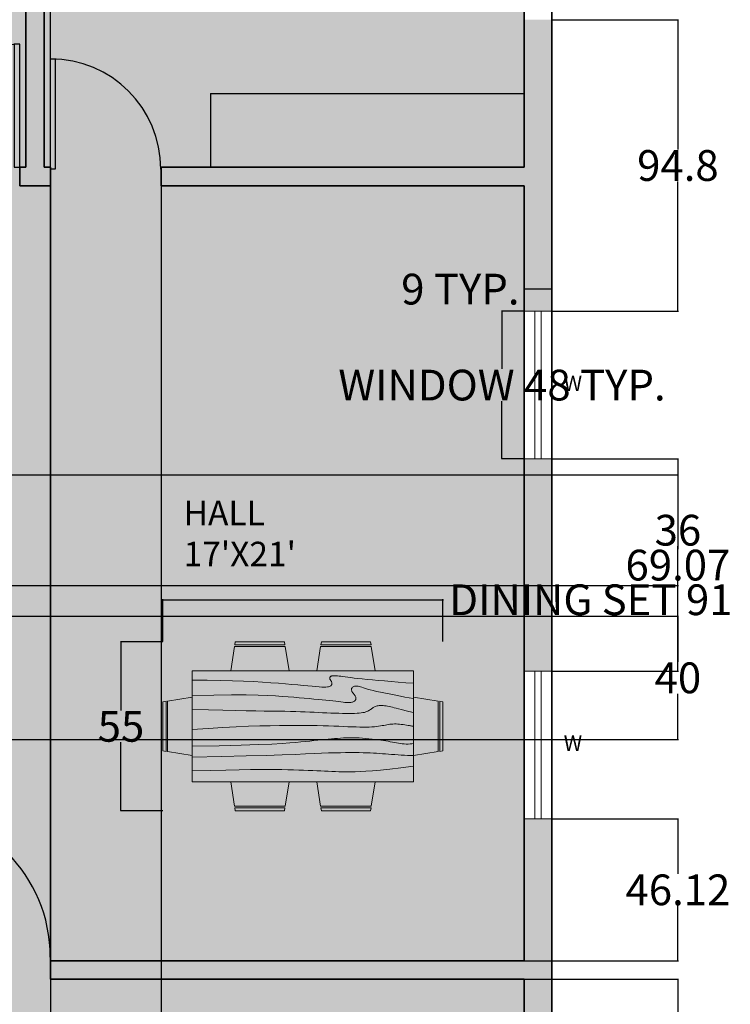
# Model space of a CAD drawing. Units: inches. Extents: x 286 to 756, y 360 to 1175.
# Tile 3 of 4: x 525 to 756, y 649 to 969. Entities that reach past the tile are written whole.
import ezdxf

# ---------------------------------------------------------------- set-up
doc = ezdxf.new("R2010")
doc.units = ezdxf.units.IN
doc.header["$MEASUREMENT"] = 0
for name, color, linetype, lineweight in [('A-ANNO-DIMS', 2, 'Continuous', 18), ('A-ANNO-TEXT', 7, 'Continuous', 18), ('A-AREA-IDEN', 7, 'Continuous', 18), ('A-FLOR-CASE', 8, 'Continuous', 25), ('A-GLAZ', 4, 'Continuous', 18), ('A-WALL', 7, 'Continuous', 35), ('DOOR', 6, 'Continuous', 25), ('FUR', 8, 'Continuous', 18)]:
    doc.layers.add(name, color=color, linetype=linetype, lineweight=lineweight)
for name, color, linetype, lineweight, true_color in [('A-FLOR-CASE-PATT', 30, 'Continuous', 13, 0xf8991e), ('A-FLOR-PATT', 9, 'Continuous', 13, 0xc7c8ca), ('A-WALL-PATT', 18, 'Continuous', 13, 0x000000)]:
    doc.layers.add(name, color=color, linetype=linetype, lineweight=lineweight, true_color=true_color)
doc.styles.get("Standard").update_dxf_attribs({"font": 'arial.ttf'})
doc.dimstyles.get("Standard").update_dxf_attribs({"dimtxt": 10, "dimasz": 0.18, "dimexe": 0.18, "dimexo": 0.0625, "dimgap": 0.09, "dimtad": 0, "dimtih": 1, "dimtoh": 1, "dimdec": 0, "dimzin": 0, "dimdsep": 46, "dimlunit": 3, "dimtxsty": 'Standard', "dimcen": 0.09, "dimadec": 0, "dimazin": 0, "dimtfac": 1, "dimtdec": 0, "dimtofl": 0, "dimtmove": 0, "dimatfit": 3, "dimfxl": 1, "dimtolj": 1, "dimtzin": 0, "dimarcsym": 0})

# ---------------------------------------------------------------- blocks, each defined once
blk = doc.blocks.new('Dining Set - 36 x 72 in.')
for p, q in [((-22.2343, 26.00059), (-23.4847, 17.99762)), ((-22.2304, 26), (-5.7608, 26)), ((-22, 27.5), (-22.1562, 26.50042)), ((-5.8416, 26.5), (-22.1534, 26.5)), ((-22, 27.5), (-6, 27.5)), ((-5.8437, 26.49966), (-6, 27.5)), ((-4.5152, 17.99762), (-5.7655, 25.99926)), ((5.7657, 26.00059), (4.5153, 17.99762)), ((5.7696, 26), (22.2392, 26)), ((6, 27.5), (5.8438, 26.50042)), ((22.1584, 26.5), (5.8466, 26.5)), ((6, 27.5), (22, 27.5)), ((22.1563, 26.49966), (22, 27.5)), ((23.4848, 17.99762), (22.2345, 25.99926)), ((36, 18), (-36, 18)), ((-36, 18), (-36, -18)), ((36, -18), (36, 18)), ((-45.5, 8), (-44.5004, 8.15617)), ((-45.5, 8), (-45.5, -8)), ((-44.5, -8.15843), (-44.5, 8.15338)), ((-44.0006, 8.23428), (-35.9976, 9.48474)), ((-44, 8.23041), (-44, -8.23915)), ((44.0006, 8.23428), (35.9976, 9.48474)), ((44, 8.23041), (44, -8.23915)), ((44.5, -8.15843), (44.5, 8.15338)), ((45.5, 8), (44.5005, 8.15617)), ((45.5, 8), (45.5, -8)), ((-44.4997, -8.15631), (-45.5, -8)), ((-35.9976, -9.48476), (-43.9993, -8.2345)), ((35.9976, -9.48476), (43.9993, -8.2345)), ((44.4997, -8.15631), (45.5, -8)), ((-36, -18), (36, -18)), ((-22.2343, -26.0006), (-23.4847, -17.99762)), ((-4.5152, -17.99762), (-5.7655, -25.99928)), ((5.7657, -26.0006), (4.5153, -17.99762)), ((23.4848, -17.99762), (22.2345, -25.99928)), ((-22.2304, -26), (-5.7608, -26)), ((-22, -27.5), (-22.1562, -26.50044)), ((-5.8416, -26.5), (-22.1534, -26.5)), ((-22, -27.5), (-6, -27.5)), ((-5.8437, -26.49967), (-6, -27.5)), ((5.7696, -26), (22.2392, -26)), ((6, -27.5), (5.8438, -26.50044)), ((22.1584, -26.5), (5.8466, -26.5)), ((6, -27.5), (22, -27.5)), ((22.1563, -26.49967), (22, -27.5))]:
    blk.add_line(p, q)
for points in [[(-36, 15), (-31.1772, 14.97754), (-26.8079, 14.91406), (-22.8538, 14.81543), (-19.276, 14.6875), (-16.0362, 14.53613), (-13.0957, 14.36718), (-10.4159, 14.18652), (-7.9583, 14), (-5.6904, 13.81315), (-3.6035, 13.63021), (-1.6954, 13.45508), (0.0365, 13.29166), (1.5945, 13.14388), (2.9811, 13.01562), (4.1988, 12.9108), (5.25, 12.83333), (6.1393, 12.78613), (6.8802, 12.76823), (7.4883, 12.77767), (7.9792, 12.8125), (8.3685, 12.87077), (8.6719, 12.95052), (8.9049, 13.0498), (9.0833, 13.16666), (9.2205, 13.29899), (9.3216, 13.44401), (9.3895, 13.59879), (9.4271, 13.76041), (9.4373, 13.92594), (9.4232, 14.09245), (9.3875, 14.257), (9.3333, 14.41666), (9.2638, 14.56917), (9.1836, 14.71484), (9.0975, 14.85465), (9.0104, 14.98958), (8.9272, 15.1206), (8.8529, 15.2487), (8.7922, 15.37483), (8.75, 15.5), (8.7305, 15.62467), (8.7344, 15.74739), (8.7617, 15.86621), (8.8125, 15.97916), (8.8867, 16.08431), (8.9844, 16.17968), (9.1055, 16.26334), (9.25, 16.33333), (9.4189, 16.38802), (9.6172, 16.42708), (9.8506, 16.45052), (10.125, 16.45833), (10.4463, 16.45052), (10.8203, 16.42708), (11.2529, 16.38802), (11.75, 16.33333), (12.3184, 16.26318), (12.9694, 16.17838), (13.7151, 16.07991), (14.5677, 15.96875), (15.5395, 15.84586), (16.6426, 15.71224), (17.8893, 15.56884), (19.2917, 15.41666), (20.859, 15.25667), (22.5879, 15.08984), (24.4721, 14.91715), (26.5052, 14.73958), (28.6809, 14.5581), (30.9929, 14.3737), (33.4347, 14.18733), (36, 14)], [(-36, 10), (-28.9766, 10.14274), (-23.1725, 10.20442), (-18.4241, 10.19775), (-14.5677, 10.13541), (-11.4399, 10.03011), (-8.877, 9.89453), (-6.7154, 9.74137), (-4.7917, 9.58333), (-2.9698, 9.43082), (-1.2246, 9.28515), (0.4415, 9.14534), (2.026, 9.01041), (3.5266, 8.87939), (4.9408, 8.7513), (6.266, 8.62516), (7.5, 8.5), (8.6411, 8.37549), (9.6914, 8.2539), (10.6538, 8.13818), (11.5312, 8.03125), (12.3267, 7.93603), (13.043, 7.85547), (13.6831, 7.79248), (14.25, 7.75), (14.7471, 7.7303), (15.1797, 7.73307), (15.5537, 7.75732), (15.875, 7.80208), (16.1494, 7.86637), (16.3828, 7.94922), (16.5811, 8.04964), (16.75, 8.16666), (16.8944, 8.29915), (17.0143, 8.44531), (17.1089, 8.60319), (17.1771, 8.77083), (17.218, 8.94629), (17.2305, 9.1276), (17.2137, 9.31282), (17.1667, 9.5), (17.0895, 9.6875), (16.987, 9.875), (16.8649, 10.0625), (16.7292, 10.25), (16.5856, 10.4375), (16.4401, 10.625), (16.2985, 10.8125), (16.1667, 11), (16.05, 11.18733), (15.9518, 11.3737), (15.8752, 11.5581), (15.8229, 11.73958), (15.798, 11.91715), (15.8034, 12.08984), (15.842, 12.25667), (15.9167, 12.41666), (16.0295, 12.56836), (16.1784, 12.70833), (16.3605, 12.83268), (16.5729, 12.9375), (16.8127, 13.01888), (17.0768, 13.07291), (17.3625, 13.0957), (17.6667, 13.08333), (17.9894, 13.03312), (18.3418, 12.94726), (18.7382, 12.82918), (19.1927, 12.68229), (19.7195, 12.51001), (20.3327, 12.31575), (21.0465, 12.10294), (21.875, 11.875), (22.8357, 11.63354), (23.959, 11.37304), (25.2786, 11.08618), (26.8282, 10.76562), (28.6414, 10.40405), (30.752, 9.99414), (33.1936, 9.52856), (36, 9)], [(-36, 5.5), (-30.7157, 5.3348), (-26.069, 5.20963), (-21.9946, 5.11767), (-18.4271, 5.05208), (-15.3009, 5.00602), (-12.5508, 4.97265), (-10.1112, 4.94515), (-7.9167, 4.91666), (-5.909, 4.88167), (-4.0586, 4.83984), (-2.3429, 4.79215), (-0.7396, 4.73958), (0.7739, 4.6831), (2.22, 4.6237), (3.6213, 4.56233), (5, 4.5), (6.373, 4.43782), (7.7344, 4.3776), (9.0723, 4.32129), (10.375, 4.27083), (11.6309, 4.22819), (12.8281, 4.19531), (13.9551, 4.17415), (15, 4.16666), (15.954, 4.17448), (16.819, 4.19791), (17.6001, 4.23698), (18.3021, 4.29166), (18.9299, 4.36198), (19.4883, 4.44791), (19.9823, 4.54948), (20.4167, 4.66666), (20.7969, 4.79899), (21.1302, 4.94401), (21.4245, 5.09879), (21.6875, 5.26041), (21.9271, 5.42594), (22.1511, 5.59245), (22.3672, 5.757), (22.5834, 5.91666), (22.8065, 6.06868), (23.0404, 6.21093), (23.2879, 6.34147), (23.5521, 6.45833), (23.8358, 6.55957), (24.142, 6.64323), (24.4735, 6.70735), (24.8334, 6.75), (25.2235, 6.76969), (25.642, 6.76692), (26.0858, 6.74267), (26.5521, 6.69791), (27.0379, 6.63362), (27.5404, 6.55078), (28.0565, 6.45036), (28.5834, 6.33333), (29.1242, 6.19987), (29.7071, 6.04687), (30.3661, 5.87044), (31.1354, 5.66666), (32.0493, 5.43164), (33.142, 5.16146), (34.4475, 4.85221), (36, 4.5)], [(-36, -1), (-30.7915, -0.6591), (-26.0195, -0.38216), (-21.6519, -0.16284), (-17.6563, 0.00521), (-14.0005, 0.12833), (-10.6523, 0.21289), (-7.5796, 0.26522), (-4.75, 0.29166), (-2.134, 0.29793), (0.2878, 0.28711), (2.5317, 0.26163), (4.6146, 0.22396), (6.5529, 0.17651), (8.3633, 0.12174), (10.0623, 0.06209), (11.6667, 0), (13.1899, -0.06201), (14.6341, -0.1211), (15.9982, -0.17432), (17.2813, -0.21875), (18.4823, -0.25147), (19.6003, -0.26953), (20.6343, -0.27002), (21.5834, -0.25), (22.4481, -0.20768), (23.2357, -0.14584), (23.9549, -0.06836), (24.6146, 0.02083), (25.2235, 0.11784), (25.7904, 0.21875), (26.3241, 0.31966), (26.8334, 0.41666), (27.3265, 0.50618), (27.8099, 0.58593), (28.2894, 0.65397), (28.7709, 0.70833), (29.2601, 0.74707), (29.763, 0.76823), (30.2855, 0.76985), (30.8334, 0.75), (31.4088, 0.70784), (31.9994, 0.64713), (32.589, 0.57275), (33.1615, 0.48958), (33.7008, 0.4025), (34.1908, 0.3164), (34.6153, 0.23616), (34.9584, 0.16666), (35.2099, 0.11165), (35.3848, 0.07031), (35.504, 0.04069), (35.5886, 0.02083), (35.6594, 0.00879), (35.7377, 0.0026), (35.8442, 0.00032), (36, 0)], [(-36, -6.5), (-27.1843, -6.31267), (-20.084, -6.1263), (-14.469, -5.9419), (-10.1094, -5.76042), (-6.7752, -5.58285), (-4.2363, -5.41016), (-2.2629, -5.24333), (-0.625, -5.08334), (0.8708, -4.93099), (2.2715, -4.78646), (3.5872, -4.64974), (4.8281, -4.52084), (6.0046, -4.39974), (7.127, -4.28646), (8.2053, -4.18099), (9.25, -4.08334), (10.2705, -3.99382), (11.2734, -3.91407), (12.2647, -3.84603), (13.25, -3.79167), (14.2354, -3.75293), (15.2266, -3.73177), (16.2295, -3.73015), (17.25, -3.75), (18.2912, -3.79248), (19.3451, -3.85547), (20.4009, -3.93604), (21.4479, -4.03125), (22.4754, -4.13819), (23.4727, -4.25391), (24.4289, -4.37549), (25.3334, -4.5), (26.1785, -4.62492), (26.9694, -4.74935), (27.7145, -4.87281), (28.4219, -4.99479), (29.1, -5.11483), (29.7572, -5.23242), (30.4016, -5.34709), (31.0417, -5.45834), (31.6837, -5.56437), (32.3262, -5.65821), (32.9658, -5.73153), (33.599, -5.77604), (34.2224, -5.78345), (34.8327, -5.74545), (35.4264, -5.65373), (36, -5.5)], [(-36, -10), (-26.4022, -9.81299), (-18.4675, -9.62891), (-11.9839, -9.45069), (-6.7396, -9.28125), (-2.5226, -9.12354), (0.8789, -8.98047), (3.6769, -8.85498), (6.0833, -8.75), (8.2767, -8.66765), (10.3021, -8.60677), (12.1712, -8.56543), (13.8958, -8.54167), (15.4876, -8.53353), (16.9583, -8.53907), (18.3197, -8.55632), (19.5834, -8.58334), (20.7616, -8.61841), (21.8685, -8.66081), (22.9188, -8.71004), (23.9271, -8.76563), (24.9081, -8.82707), (25.8763, -8.89388), (26.8465, -8.96558), (27.8334, -9.04167), (28.8474, -9.12118), (29.8828, -9.20117), (30.93, -9.27824), (31.9792, -9.34896), (33.0205, -9.40991), (34.0443, -9.45768), (35.0407, -9.48885), (36, -9.5)], [(-36, -14.5), (-30.0881, -14.33513), (-25.0332, -14.21224), (-20.7312, -14.12647), (-17.0781, -14.07292), (-13.97, -14.04671), (-11.3027, -14.04297), (-8.9724, -14.05681), (-6.875, -14.08334), (-4.9224, -14.11833), (-3.0905, -14.16016), (-1.3709, -14.20785), (0.2448, -14.26042), (1.7647, -14.3169), (3.1973, -14.3763), (4.5507, -14.43767), (5.8333, -14.5), (7.0554, -14.5621), (8.235, -14.62175), (9.3922, -14.67652), (10.5469, -14.72396), (11.7192, -14.76164), (12.929, -14.78711), (14.1965, -14.79794), (15.5417, -14.79167), (16.9933, -14.76424), (18.6152, -14.70508), (20.4804, -14.60197), (22.6615, -14.44271), (25.2312, -14.21509), (28.2624, -13.9069), (31.8277, -13.50594), (36, -13)]]:
    blk.add_lwpolyline(points)
blk = doc.blocks.new('*U7')
for p, q in [((0, 0), (0, -6)), ((-40, 0), (-40, -6))]:
    blk.add_line(p, q)
blk.add_lwpolyline([(0, 0), (0, 40), (-1.75, 40), (-1.75, 0)], close=True)
blk.add_arc((0, 0), 40, 90, 180)
blk = doc.blocks.new('*U2')
for p, q in [((0, 0), (0, -6)), ((40, 0), (40, -6))]:
    blk.add_line(p, q)
blk.add_lwpolyline([(0, 0), (0, 40), (1.75, 40), (1.75, 0)], close=True)
blk.add_arc((0, 0), 40, 0, 90)
blk = doc.blocks.new('*U8')
for p, q in [((0, 0), (0, -6)), ((40, 0), (40, -6))]:
    blk.add_line(p, q)
blk.add_lwpolyline([(0, 0), (0, 40), (1.75, 40), (1.75, 0)], close=True)
blk.add_arc((0, 0), 40, 0, 90)
blk = doc.blocks.new('WIN-48IN-WALL9')
for p, q in [((9, 48), (0, 48)), ((3.5, 0), (3.5, 48)), ((5.5, 0), (5.5, 48)), ((9, 0), (0, 0))]:
    blk.add_line(p, q)
blk = doc.blocks.new('*D13')
at = {"layer": 'A-ANNO-DIMS', "color": 0, "lineweight": -2, "transparency": 16777216}
for p, q in [((688.8, 873.95), (681.49, 873.95)), ((681.67, 873.77), (681.67, 855.21)), ((681.67, 826.13), (681.67, 844.68)), ((688.8, 825.95), (681.49, 825.95))]:
    blk.add_line(p, q, dxfattribs=at)
at = {"layer": 'A-ANNO-DIMS', "color": 0, "transparency": 16777216}
for points in [[(681.64, 873.77), (681.7, 873.77), (681.67, 873.95)], [(681.64, 826.13), (681.7, 826.13), (681.67, 825.95)]]:
    blk.add_solid(points, dxfattribs=at)
at = {"layer": 'Defpoints', "color": 0, "transparency": 16777216}
for p in [(688.87, 873.95), (681.67, 825.95), (688.87, 825.95)]:
    blk.add_point(p, dxfattribs=at)
at = {"layer": 'A-ANNO-DIMS', "color": 0, "transparency": 16777216, "insert": (681.67, 849.95), "char_height": 10, "attachment_point": 5}
blk.add_mtext('\\A1;WINDOW 48 TYP.', dxfattribs=at)
blk = doc.blocks.new('*D14')
at = {"layer": 'A-ANNO-DIMS', "color": 0, "lineweight": -2, "transparency": 16777216}
for p, q in [((688.87, 881.15), (688.69, 881.15)), ((688.87, 874.01), (688.87, 881.33)), ((697.69, 881.15), (689.05, 881.15)), ((697.87, 874.01), (697.87, 881.33))]:
    blk.add_line(p, q, dxfattribs=at)
at = {"layer": 'A-ANNO-DIMS', "color": 0, "transparency": 16777216}
for points in [[(689.05, 881.18), (689.05, 881.12), (688.87, 881.15)], [(697.69, 881.18), (697.69, 881.12), (697.87, 881.15)]]:
    blk.add_solid(points, dxfattribs=at)
at = {"layer": 'Defpoints', "color": 0, "transparency": 16777216}
for p in [(688.87, 881.15), (688.87, 873.95), (697.87, 873.95)]:
    blk.add_point(p, dxfattribs=at)
at = {"layer": 'A-ANNO-DIMS', "color": 0, "transparency": 16777216, "insert": (668.14, 881.15), "char_height": 10, "attachment_point": 5}
blk.add_mtext('\\A1;9 TYP.', dxfattribs=at)
blk = doc.blocks.new('*D17')
at = {"layer": 'A-ANNO-DIMS', "color": 0, "lineweight": -2, "transparency": 16777216}
for p, q in [((571.44, 766.55), (571.44, 780.32)), ((571.62, 780.14), (662.26, 780.14)), ((662.44, 766.55), (662.44, 780.32)), ((662.44, 780.14), (662.62, 780.14))]:
    blk.add_line(p, q, dxfattribs=at)
at = {"layer": 'A-ANNO-DIMS', "color": 0, "transparency": 16777216}
for points in [[(571.62, 780.17), (571.62, 780.11), (571.44, 780.14)], [(662.26, 780.17), (662.26, 780.11), (662.44, 780.14)]]:
    blk.add_solid(points, dxfattribs=at)
at = {"layer": 'Defpoints', "color": 0, "transparency": 16777216}
for p in [(662.44, 780.14), (571.44, 766.49), (662.44, 766.49)]:
    blk.add_point(p, dxfattribs=at)
at = {"layer": 'A-ANNO-DIMS', "color": 0, "transparency": 16777216, "insert": (710.58, 780.14), "char_height": 10, "attachment_point": 5}
blk.add_mtext('\\A1;DINING SET 91', dxfattribs=at)
blk = doc.blocks.new('*D18')
at = {"layer": 'A-ANNO-DIMS', "color": 0, "lineweight": -2, "transparency": 16777216}
for p, q in [((571.38, 766.49), (557.61, 766.49)), ((557.79, 766.31), (557.79, 744.17)), ((557.79, 711.67), (557.79, 733.82)), ((571.38, 711.49), (557.61, 711.49))]:
    blk.add_line(p, q, dxfattribs=at)
at = {"layer": 'A-ANNO-DIMS', "color": 0, "transparency": 16777216}
for points in [[(557.76, 766.31), (557.82, 766.31), (557.79, 766.49)], [(557.76, 711.67), (557.82, 711.67), (557.79, 711.49)]]:
    blk.add_solid(points, dxfattribs=at)
at = {"layer": 'Defpoints', "color": 0, "transparency": 16777216}
for p in [(557.79, 766.49), (571.44, 766.49), (571.44, 711.49)]:
    blk.add_point(p, dxfattribs=at)
at = {"layer": 'A-ANNO-DIMS', "color": 0, "transparency": 16777216, "insert": (557.79, 738.99), "char_height": 10, "attachment_point": 5}
blk.add_mtext('\\A1;55', dxfattribs=at)
blk = doc.blocks.new('*D25')
at = {"layer": 'A-ANNO-DIMS', "color": 0, "lineweight": -2, "transparency": 16777216}
for p, q in [((688.93, 656.76), (739.05, 656.76)), ((738.87, 656.58), (738.87, 537.45)), ((738.87, 407.94), (738.87, 527.06)), ((697.93, 407.76), (739.05, 407.76))]:
    blk.add_line(p, q, dxfattribs=at)
at = {"layer": 'A-ANNO-DIMS', "color": 0, "transparency": 16777216}
for points in [[(738.84, 656.58), (738.9, 656.58), (738.87, 656.76)], [(738.84, 407.94), (738.9, 407.94), (738.87, 407.76)]]:
    blk.add_solid(points, dxfattribs=at)
at = {"layer": 'Defpoints', "color": 0, "transparency": 16777216}
for p in [(688.87, 656.76), (738.87, 656.76), (697.87, 407.76)]:
    blk.add_point(p, dxfattribs=at)
at = {"layer": 'A-ANNO-DIMS', "color": 0, "transparency": 16777216, "insert": (738.87, 532.26), "char_height": 10, "attachment_point": 5}
blk.add_mtext('\\A1;249', dxfattribs=at)
blk = doc.blocks.new('*D27')
at = {"layer": 'A-ANNO-DIMS', "color": 0, "lineweight": -2, "transparency": 16777216}
for p, q in [((486.87, 656.82), (486.87, 1168.94)), ((487.05, 1168.76), (503.4, 1168.76)), ((534.69, 1168.76), (518.33, 1168.76)), ((534.87, 656.82), (534.87, 1168.94))]:
    blk.add_line(p, q, dxfattribs=at)
at = {"layer": 'A-ANNO-DIMS', "color": 0, "transparency": 16777216}
for points in [[(487.05, 1168.79), (487.05, 1168.73), (486.87, 1168.76)], [(534.69, 1168.79), (534.69, 1168.73), (534.87, 1168.76)]]:
    blk.add_solid(points, dxfattribs=at)
at = {"layer": 'Defpoints', "color": 0, "transparency": 16777216}
for p in [(534.87, 1168.76), (486.87, 656.76), (534.87, 656.76)]:
    blk.add_point(p, dxfattribs=at)
at = {"layer": 'A-ANNO-DIMS', "color": 0, "transparency": 16777216, "insert": (510.87, 1168.76), "char_height": 10, "attachment_point": 5}
blk.add_mtext('\\A1;48', dxfattribs=at)
blk = doc.blocks.new('*D28')
at = {"layer": 'A-ANNO-DIMS', "color": 0, "lineweight": -2, "transparency": 16777216}
for p, q in [((697.93, 708.88), (739.05, 708.88)), ((738.87, 708.7), (738.87, 691.01)), ((738.87, 662.94), (738.87, 680.62)), ((688.93, 662.76), (739.05, 662.76))]:
    blk.add_line(p, q, dxfattribs=at)
at = {"layer": 'A-ANNO-DIMS', "color": 0, "transparency": 16777216}
for points in [[(738.84, 708.7), (738.9, 708.7), (738.87, 708.88)], [(738.84, 662.94), (738.9, 662.94), (738.87, 662.76)]]:
    blk.add_solid(points, dxfattribs=at)
at = {"layer": 'Defpoints', "color": 0, "transparency": 16777216}
for p in [(697.87, 708.88), (738.87, 708.88), (688.87, 662.76)]:
    blk.add_point(p, dxfattribs=at)
at = {"layer": 'A-ANNO-DIMS', "color": 0, "transparency": 16777216, "insert": (738.87, 685.82), "char_height": 10, "attachment_point": 5}
blk.add_mtext('\\A1;46.12', dxfattribs=at)
blk = doc.blocks.new('*D29')
at = {"layer": 'A-ANNO-DIMS', "color": 0, "lineweight": -2, "transparency": 16777216}
for p, q in [((697.93, 825.95), (739.05, 825.95)), ((738.87, 825.77), (738.87, 796.61)), ((738.87, 757.06), (738.87, 786.22)), ((697.93, 756.88), (739.05, 756.88))]:
    blk.add_line(p, q, dxfattribs=at)
at = {"layer": 'A-ANNO-DIMS', "color": 0, "transparency": 16777216}
for points in [[(738.84, 825.77), (738.9, 825.77), (738.87, 825.95)], [(738.84, 757.06), (738.9, 757.06), (738.87, 756.88)]]:
    blk.add_solid(points, dxfattribs=at)
at = {"layer": 'Defpoints', "color": 0, "transparency": 16777216}
for p in [(697.87, 825.95), (738.87, 825.95), (697.87, 756.88)]:
    blk.add_point(p, dxfattribs=at)
at = {"layer": 'A-ANNO-DIMS', "color": 0, "transparency": 16777216, "insert": (738.87, 791.41), "char_height": 10, "attachment_point": 5}
blk.add_mtext('\\A1;69.07', dxfattribs=at)
blk = doc.blocks.new('*D30')
at = {"layer": 'A-ANNO-DIMS', "color": 0, "lineweight": -2, "transparency": 16777216}
for p, q in [((697.93, 968.76), (739.05, 968.76)), ((738.87, 968.58), (738.87, 926.55)), ((738.87, 874.13), (738.87, 916.16)), ((697.93, 873.95), (739.05, 873.95))]:
    blk.add_line(p, q, dxfattribs=at)
at = {"layer": 'A-ANNO-DIMS', "color": 0, "transparency": 16777216}
for points in [[(738.84, 968.58), (738.9, 968.58), (738.87, 968.76)], [(738.84, 874.13), (738.9, 874.13), (738.87, 873.95)]]:
    blk.add_solid(points, dxfattribs=at)
at = {"layer": 'Defpoints', "color": 0, "transparency": 16777216}
for p in [(697.87, 968.76), (738.87, 968.76), (697.87, 873.95)]:
    blk.add_point(p, dxfattribs=at)
at = {"layer": 'A-ANNO-DIMS', "color": 0, "transparency": 16777216, "insert": (738.87, 921.35), "char_height": 10, "attachment_point": 5}
blk.add_mtext('\\A1;94.8', dxfattribs=at)
blk = doc.blocks.new('*D37')
at = {"layer": 'A-ANNO-DIMS', "color": 0, "lineweight": -2, "transparency": 16777216}
for p, q in [((478.93, 774.76), (739.05, 774.76)), ((738.87, 774.58), (738.87, 759.95)), ((738.87, 734.94), (738.87, 749.56)), ((478.93, 734.76), (739.05, 734.76))]:
    blk.add_line(p, q, dxfattribs=at)
at = {"layer": 'A-ANNO-DIMS', "color": 0, "transparency": 16777216}
for points in [[(738.84, 774.58), (738.9, 774.58), (738.87, 774.76)], [(738.84, 734.94), (738.9, 734.94), (738.87, 734.76)]]:
    blk.add_solid(points, dxfattribs=at)
at = {"layer": 'Defpoints', "color": 0, "transparency": 16777216}
for p in [(478.87, 774.76), (738.87, 774.76), (478.87, 734.76)]:
    blk.add_point(p, dxfattribs=at)
at = {"layer": 'A-ANNO-DIMS', "color": 0, "transparency": 16777216, "insert": (738.87, 754.76), "char_height": 10, "attachment_point": 5}
blk.add_mtext('\\A1;40', dxfattribs=at)
blk = doc.blocks.new('*D38')
at = {"layer": 'A-ANNO-DIMS', "color": 0, "lineweight": -2, "transparency": 16777216}
for p, q in [((478.93, 820.76), (739.05, 820.76)), ((738.87, 820.58), (738.87, 807.95)), ((738.87, 784.94), (738.87, 797.56)), ((478.93, 784.76), (739.05, 784.76))]:
    blk.add_line(p, q, dxfattribs=at)
at = {"layer": 'A-ANNO-DIMS', "color": 0, "transparency": 16777216}
for points in [[(738.84, 820.58), (738.9, 820.58), (738.87, 820.76)], [(738.84, 784.94), (738.9, 784.94), (738.87, 784.76)]]:
    blk.add_solid(points, dxfattribs=at)
at = {"layer": 'Defpoints', "color": 0, "transparency": 16777216}
for p in [(478.87, 820.76), (738.87, 820.76), (478.87, 784.76)]:
    blk.add_point(p, dxfattribs=at)
at = {"layer": 'A-ANNO-DIMS', "color": 0, "transparency": 16777216, "insert": (738.87, 802.76), "char_height": 10, "attachment_point": 5}
blk.add_mtext('\\A1;36', dxfattribs=at)
blk = doc.blocks.new('*D40')
at = {"layer": 'A-ANNO-DIMS', "color": 0, "lineweight": -2, "transparency": 16777216}
for p, q in [((534.87, 920.69), (534.87, 366.58)), ((570.87, 920.69), (570.87, 366.58)), ((535.05, 366.76), (545.62, 366.76)), ((570.69, 366.76), (560.11, 366.76))]:
    blk.add_line(p, q, dxfattribs=at)
at = {"layer": 'A-ANNO-DIMS', "color": 0, "transparency": 16777216}
for points in [[(535.05, 366.79), (535.05, 366.73), (534.87, 366.76)], [(570.69, 366.79), (570.69, 366.73), (570.87, 366.76)]]:
    blk.add_solid(points, dxfattribs=at)
at = {"layer": 'Defpoints', "color": 0, "transparency": 16777216}
for p in [(534.87, 920.76), (570.87, 920.76), (570.87, 366.76)]:
    blk.add_point(p, dxfattribs=at)
at = {"layer": 'A-ANNO-DIMS', "color": 0, "transparency": 16777216, "insert": (552.87, 366.76), "char_height": 10, "attachment_point": 5}
blk.add_mtext('\\A1;36', dxfattribs=at)

msp = doc.modelspace()

# ---------------------------------------------------------------- hatches: boundary and pattern name
at = {"layer": 'A-FLOR-CASE-PATT'}
h = msp.add_hatch(color=256, dxfattribs=at)
h.dxf.hatch_style = 1
h.paths.add_polyline_path([(448.865, 944.756), (346.865, 944.756), (346.865, 920.756), (448.865, 920.756)])
h.paths.add_polyline_path([(478.865, 914.756), (454.865, 914.756), (454.865, 844.756), (478.865, 844.756)])
h.paths.add_polyline_path([(688.865, 944.756), (586.865, 944.756), (586.865, 920.756), (688.865, 920.756)])
at = {"layer": 'A-FLOR-PATT'}
h = msp.add_hatch(color=256, dxfattribs=at)
h.dxf.hatch_style = 1
h.paths.add_polyline_path([(526.865, 1064.756), (386.892, 1064.756), (346.865, 1064.756), (346.865, 944.756), (448.865, 944.756), (448.865, 920.756), (484.865, 920.756), (484.865, 914.756), (524.865, 914.756), (524.865, 920.756), (526.865, 920.756)])
h.paths.add_polyline_path([(418.865, 1118.756), (346.865, 1118.756), (346.865, 1070.756), (386.865, 1070.756), (386.865, 1064.756), (386.892, 1064.756), (416.865, 1064.756), (416.865, 1070.756), (418.865, 1070.756)])
h.paths.add_polyline_path([(526.865, 1118.756), (424.865, 1118.756), (424.865, 1070.756), (494.865, 1070.756), (494.865, 1064.756), (524.865, 1064.756), (524.865, 1070.756), (526.865, 1070.756)])
h.paths.add_polyline_path([(610.865, 1118.756), (532.865, 1118.756), (532.865, 1070.756), (534.865, 1070.756), (534.865, 1064.756), (564.865, 1064.756), (564.865, 1070.756), (610.865, 1070.756)])
h.paths.add_polyline_path([(688.865, 1118.756), (616.865, 1118.756), (616.865, 1070.756), (618.865, 1070.756), (618.865, 1064.756), (648.865, 1064.756), (648.865, 1070.756), (688.865, 1070.756)])
h.paths.add_polyline_path([(688.865, 1064.756), (648.865, 1064.756), (618.865, 1064.756), (532.865, 1064.756), (532.865, 920.756), (534.865, 920.756), (534.865, 914.756), (570.865, 914.756), (570.865, 920.756), (586.865, 920.756), (586.865, 944.756), (688.865, 944.756)])
h.paths.add_polyline_path([(484.865, 820.756), (478.865, 820.756), (478.865, 844.756), (454.865, 844.756), (454.865, 914.756), (346.865, 914.756), (346.865, 782.756), (478.865, 782.756), (478.865, 784.756), (484.865, 784.756)])
h.paths.add_polyline_path([(688.865, 914.756), (570.865, 914.756), (534.865, 914.756), (484.865, 914.756), (484.865, 820.756), (484.865, 784.756), (484.865, 734.577), (484.865, 662.756), (486.865, 662.756), (486.865, 656.756), (534.865, 656.756), (534.865, 662.756), (688.865, 662.756)])
h.paths.add_polyline_path([(478.865, 734.756), (484.865, 734.756), (484.865, 774.756), (478.865, 774.756), (478.865, 776.756), (388.865, 776.756), (388.865, 734.756), (370.865, 734.756), (370.865, 686.756), (478.865, 686.756)])
h.paths.add_polyline_path([(688.865, 656.756), (534.865, 656.756), (486.865, 656.756), (484.865, 656.756), (346.865, 656.756), (346.865, 536.756), (388.865, 536.756), (388.865, 530.756), (388.865, 506.756), (388.865, 488.756), (388.865, 464.756), (388.865, 452.756), (466.865, 452.756), (466.865, 416.756), (496.865, 416.756), (544.865, 416.756), (580.865, 416.756), (688.865, 416.756)])
h.paths.add_polyline_path([(388.865, 530.756), (346.865, 530.756), (346.865, 494.756), (382.865, 494.756), (382.865, 506.756), (388.865, 506.756)], flags=17)
h.paths.add_polyline_path([(382.865, 464.756), (388.865, 464.756), (388.865, 488.756), (346.865, 488.756), (346.865, 452.756), (382.865, 452.756)], flags=17)
at = {"layer": 'A-WALL-PATT'}
h = msp.add_hatch(color=256, dxfattribs=at)
h.dxf.hatch_style = 1
h.paths.add_polyline_path([(496.865, 416.756), (346.865, 416.756), (346.865, 656.756), (484.865, 656.756), (486.865, 656.756), (486.865, 662.756), (484.865, 662.756), (484.865, 734.577), (478.865, 734.577), (478.865, 662.756), (346.865, 662.756), (346.865, 686.756), (337.865, 686.756), (337.865, 407.756), (496.865, 407.756)])
h.paths.add_polyline_path([(484.865, 784.756), (478.865, 784.756), (478.865, 782.756), (346.865, 782.756), (346.865, 914.756), (406.865, 914.756), (478.865, 914.756), (478.865, 820.756), (484.865, 820.756), (484.865, 920.756), (346.865, 920.756), (346.865, 968.756), (337.865, 968.756), (337.865, 710.756), (346.865, 710.756), (346.865, 734.756), (388.865, 734.756), (388.865, 776.756), (478.865, 776.756), (478.865, 774.756), (484.865, 774.756)])
h.paths.add_polyline_path([(382.865, 776.756), (382.865, 740.756), (346.865, 740.756), (346.865, 776.756)], flags=16)
h.paths.add_polyline_path([(386.865, 1070.756), (346.865, 1070.756), (346.865, 1118.756), (418.865, 1118.756), (418.865, 1106.756), (424.865, 1106.756), (424.865, 1118.756), (526.865, 1118.756), (526.865, 1070.756), (532.865, 1070.756), (532.865, 1118.756), (610.865, 1118.756), (610.865, 1106.756), (616.865, 1106.756), (616.865, 1118.756), (688.865, 1118.756), (688.865, 1016.756), (697.865, 1016.756), (697.865, 1127.756), (337.865, 1127.756), (337.865, 1016.756), (346.865, 1016.756), (346.865, 1030.663), (346.865, 1064.756), (386.865, 1064.756)])
h.paths.add_polyline_path([(494.822, 1069.262, -0.0124335), (494.859, 1070.756), (424.865, 1070.756), (424.865, 1082.756), (418.865, 1082.756), (418.865, 1070.756), (416.865, 1070.756), (416.865, 1069.252), (416.865, 1064.756), (494.822, 1064.756)], flags=17)
h.paths.add_polyline_path([(618.865, 1069.261), (618.865, 1070.756), (616.865, 1070.756), (616.865, 1082.756), (610.865, 1082.756), (610.865, 1070.756), (564.872, 1070.756, -0.0124335), (564.909, 1069.262), (564.909, 1064.756), (618.865, 1064.756)], flags=17)
h.paths.add_polyline_path([(688.865, 1070.756), (648.865, 1070.756), (648.865, 1070.756, -0.0124418), (648.902, 1069.261), (648.902, 1064.756), (688.865, 1064.756)], flags=17)
h.paths.add_polyline_path([(697.865, 968.756), (688.865, 968.756), (688.865, 920.756), (570.865, 920.756), (570.865, 914.756), (688.865, 914.756), (688.865, 873.949), (697.865, 873.949)])
h.paths.add_polyline_path([(697.865, 825.949), (688.865, 825.949), (688.865, 756.879), (697.865, 756.879)])
h.paths.add_polyline_path([(532.865, 1064.756), (526.865, 1064.756), (526.865, 920.756), (524.865, 920.756), (524.865, 914.756), (534.865, 914.756), (534.865, 920.756), (532.865, 920.756)])
h = msp.add_hatch(color=256, dxfattribs=at)
h.dxf.hatch_style = 1
h.paths.add_polyline_path([(697.865, 708.879), (688.865, 708.879), (688.865, 662.756), (534.865, 662.756), (534.865, 656.756), (688.865, 656.756), (688.865, 407.756), (697.865, 407.756)])
h.paths.add_polyline_path([(580.865, 416.756), (544.865, 416.756), (544.865, 407.756), (580.865, 407.756)], flags=17)

# ---------------------------------------------------------------- linework, layer by layer
at = {"layer": 'A-FLOR-CASE'}
for q in [(688.865, 944.756), (586.865, 920.756)]:
    msp.add_line((586.865, 944.756), q, dxfattribs=at)
at = {"layer": 'A-GLAZ'}
for p, q in [((697.865, 756.879), (688.865, 756.879)), ((692.365, 708.879), (692.365, 756.879)), ((694.365, 708.879), (694.365, 756.879)), ((697.865, 708.879), (688.865, 708.879))]:
    msp.add_line(p, q, dxfattribs=at)
at = {"layer": 'A-WALL'}
for p, q in [((697.865, 407.756), (697.865, 1127.756)), ((688.865, 920.756), (688.865, 1118.756)), ((526.865, 1064.756), (526.865, 920.756)), ((532.865, 1064.756), (532.865, 920.756)), ((524.865, 914.756), (524.865, 920.756)), ((524.865, 920.756), (526.865, 920.756)), ((532.865, 920.756), (534.865, 920.756)), ((534.865, 920.756), (534.865, 914.756)), ((688.865, 920.756), (570.865, 920.756)), ((570.865, 920.756), (570.865, 914.756)), ((526.865, 914.756), (524.865, 914.756)), ((532.865, 914.756), (526.865, 914.756)), ((534.865, 914.756), (532.865, 914.756)), ((688.865, 914.756), (570.865, 914.756)), ((688.865, 662.756), (688.865, 914.756)), ((534.865, 662.756), (534.865, 656.756)), ((534.865, 662.756), (688.865, 662.756)), ((534.865, 656.756), (688.865, 656.756)), ((688.865, 407.756), (688.865, 656.756))]:
    msp.add_line(p, q, dxfattribs=at)

# ---------------------------------------------------------------- block references
at = {"layer": 'A-GLAZ', "rotation": 180}
msp.add_blockref('WIN-48IN-WALL9', (697.865, 873.949), dxfattribs=at)
at = {"layer": 'DOOR'}
msp.add_blockref('*U7', (524.865, 920.756), dxfattribs=at)
for name, p, xscale, yscale, zscale in [('*U2', (534.865, 920.141), 0.897500393084551, 0.897500393084551, 0.897500393084551), ('*U8', (486.865, 663.949), 1.198937203557198, 1.198937203557198, 1.198937203557198)]:
    msp.add_blockref(name, p, dxfattribs=dict(at, xscale=xscale, yscale=yscale, zscale=zscale))
at = {"layer": 'FUR'}
msp.add_blockref('Dining Set - 36 x 72 in.', (616.944, 738.991), dxfattribs=at)

# ---------------------------------------------------------------- texts
at = {"layer": 'A-ANNO-TEXT', "char_height": 5, "attachment_point": 1}
for insert in [(701.741, 853.041), (701.741, 736.019)]:
    msp.add_mtext_dynamic_manual_height_columns('W', width=36.25002, gutter_width=1, heights=[0], dxfattribs=dict(at, insert=insert))
at = {"layer": 'A-AREA-IDEN', "insert": (578.142, 812.343), "char_height": 8, "attachment_point": 1}
msp.add_mtext_dynamic_manual_height_columns("HALL\\P17'X21'", width=59.48304, gutter_width=1, heights=[0], dxfattribs=at)

# ---------------------------------------------------------------- dimensions: what is measured, and where the dimension line sits
at = {"layer": 'A-ANNO-DIMS'}
for base, p1, p2, picture, middle in [((534.865, 1168.756), (486.865, 656.756), (534.865, 656.756), '*D27', (510.865, 1168.756)), ((570.865, 366.756), (534.865, 920.756), (570.865, 920.756), '*D40', (552.865, 366.756))]:
    dim = msp.add_linear_dim(base=base, p1=p1, p2=p2, dimstyle='Standard', override={"dimdec": 0, "dimlfac": 1, "dimrnd": 0, "dimzin": 0, "dimdsep": 46, "dimlunit": 2}, dxfattribs=at)
    dim.commit()
    dim.dimension.update_dxf_attribs({"geometry": picture, "text_midpoint": middle})
for base, p1, p2, override, picture, middle in [((738.865, 968.756), (697.865, 873.949), (697.865, 968.756), {"dimdec": 1, "dimlfac": 1, "dimrnd": 0, "dimzin": 0, "dimdsep": 46, "dimlunit": 2}, '*D30', (738.865, 921.352)), ((738.865, 825.949), (697.865, 756.879), (697.865, 825.949), {"dimdec": 2, "dimlfac": 1, "dimrnd": 0, "dimzin": 0, "dimdsep": 46, "dimlunit": 2}, '*D29', (738.865, 791.414)), ((738.865, 820.756), (478.865, 784.756), (478.865, 820.756), {"dimdec": 0, "dimlfac": 1, "dimrnd": 0, "dimzin": 0, "dimdsep": 46, "dimlunit": 2}, '*D38', (738.865, 802.756)), ((738.865, 774.756), (478.865, 734.756), (478.865, 774.756), {"dimdec": 0, "dimlfac": 1, "dimrnd": 0, "dimzin": 0, "dimdsep": 46, "dimlunit": 2}, '*D37', (738.865, 754.756)), ((557.794, 766.491), (571.444, 711.491), (571.444, 766.491), {"dimdec": 0, "dimlfac": 1, "dimrnd": 0, "dimzin": 0, "dimdsep": 46, "dimlunit": 2}, '*D18', (557.794, 738.991)), ((738.865, 708.879), (688.865, 662.756), (697.865, 708.879), {"dimdec": 2, "dimlfac": 1, "dimrnd": 0, "dimzin": 0, "dimdsep": 46, "dimlunit": 2}, '*D28', (738.865, 685.817)), ((738.865, 656.756), (697.865, 407.756), (688.865, 656.756), {"dimdec": 0, "dimlfac": 1, "dimrnd": 0, "dimzin": 0, "dimdsep": 46, "dimlunit": 2}, '*D25', (738.865, 532.256))]:
    dim = msp.add_linear_dim(base=base, p1=p1, p2=p2, angle=90, dimstyle='Standard', override=override, dxfattribs=at)
    dim.commit()
    dim.dimension.update_dxf_attribs({"geometry": picture, "text_midpoint": middle})
for base, p1, p2, angle, text, picture, middle in [((688.865, 881.149), (697.865, 873.949), (688.865, 873.949), 180, '<> TYP.', '*D14', (668.142, 881.149)), ((681.665, 825.949), (688.865, 873.949), (688.865, 825.949), 270, 'WINDOW <> TYP.', '*D13', (681.665, 849.949))]:
    dim = msp.add_linear_dim(base=base, p1=p1, p2=p2, angle=angle, text=text, dimstyle='Standard', override={"dimdec": 0, "dimlfac": 1, "dimrnd": 0, "dimzin": 0, "dimdsep": 46, "dimlunit": 2}, dxfattribs=at)
    dim.commit()
    dim.dimension.update_dxf_attribs({"geometry": picture, "text_midpoint": middle})
dim = msp.add_linear_dim(base=(662.444, 780.141), p1=(571.444, 766.491), p2=(662.444, 766.491), text='DINING SET <>', dimstyle='Standard', override={"dimdec": 0, "dimlfac": 1, "dimrnd": 0, "dimzin": 0, "dimdsep": 46, "dimlunit": 2}, dxfattribs=at)
dim.commit()
dim.dimension.update_dxf_attribs({"geometry": '*D17', "text_midpoint": (710.575, 780.141)})

doc.saveas('drawing.dxf')
